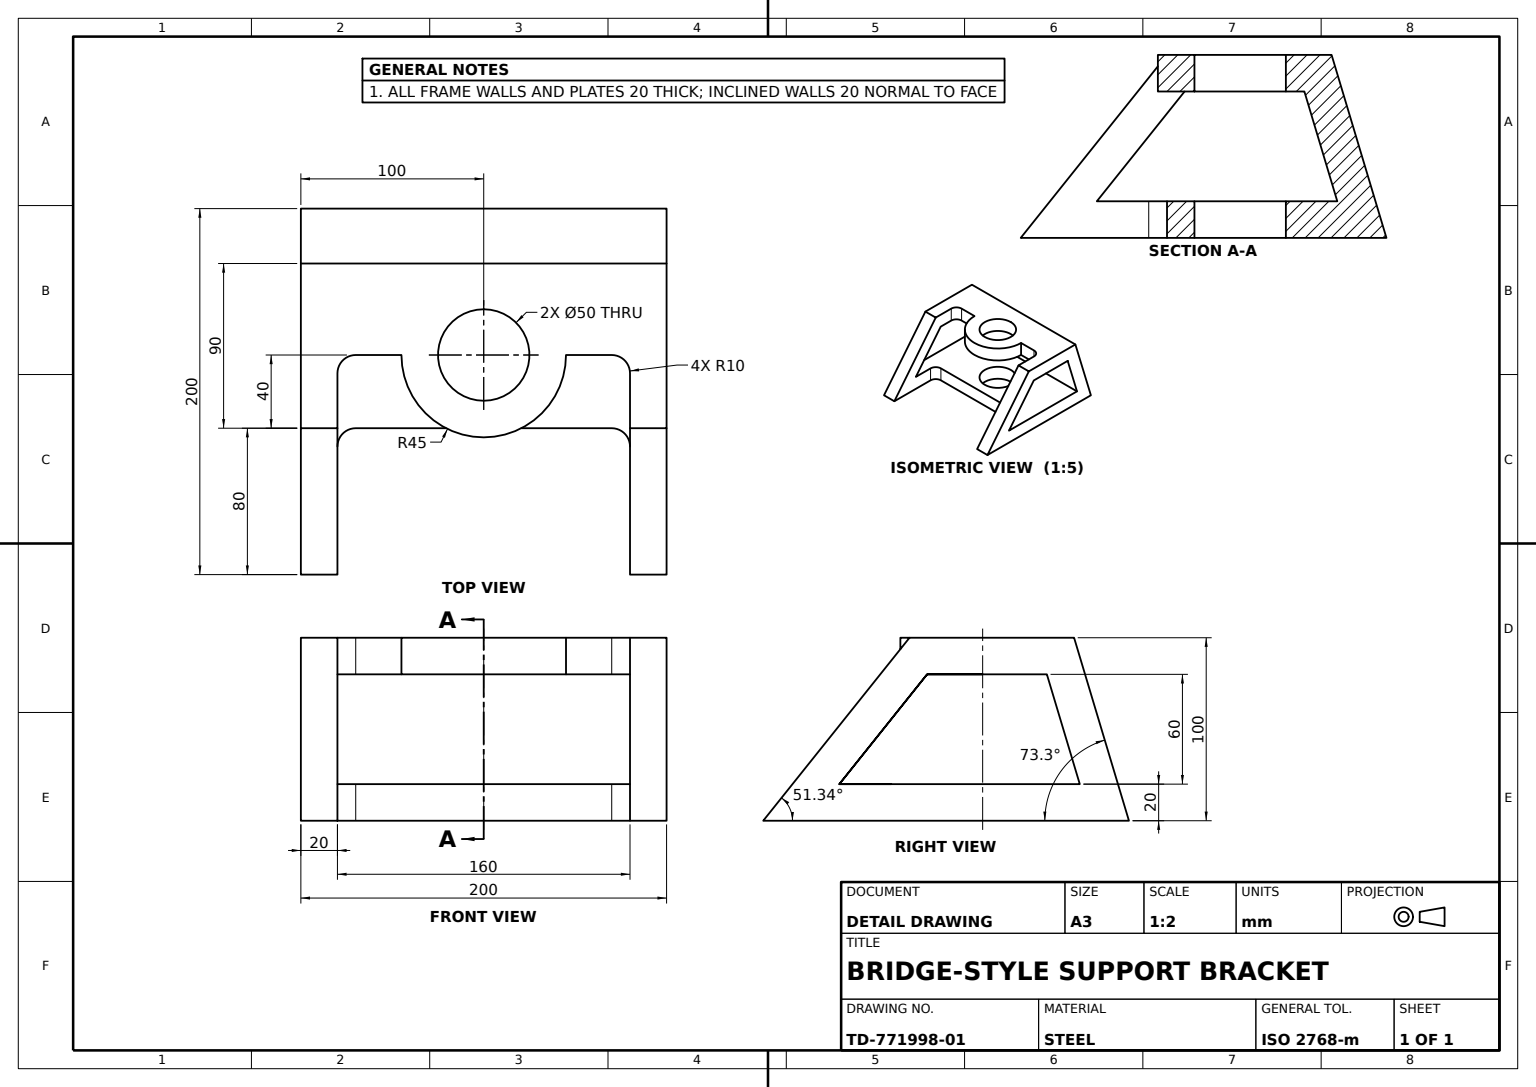
from build123d import *

# Parameters (mm, degrees)
FRAME_BODY_200_DEPTH        = 100
CENTRE_RECESS_SKETCH_W      = 160
CENTRE_RECESS_SKETCH_H      = 60
CENTRE_RECESS_CUT_DEPTH     = 150
WINDOW_A_CUT_REACH          = 246.949
WINDOW_A_SKETCH_80X60_W     = 160
WINDOW_A_SKETCH_80X60_H     = 60
WINDOW_B_CUT_REACH          = 239.487
WINDOW_B_SKETCH_W           = 160
WINDOW_B_SKETCH_H           = 80
WINDOW_CORNER_FILLETS_R10_R = 10
ANCHOR_BOSS_SKETCH_90_R     = 45
ANCHOR_BOSS_90_DEPTH        = 20
ANCHOR_BORE_SKETCH_50_R     = 25
ANCHOR_BORE_50_DEPTH        = 245.948974278


with BuildPart() as part:
    # Frame Profile Sketch → Frame Body 200 (new, symmetric)
    with BuildSketch(Plane(origin=(0, 0, 0), x_dir=(0, 0, -1), z_dir=(1, 0, 0))):
        Polygon((200, 0), (170, 100), (80, 100), (0, 0), align=None)
        Polygon((155.119386982, 80), (89.61249695, 80), (41.61249695, 20), (173.119386982, 20), align=None, mode=Mode.SUBTRACT)
    extrude(amount=FRAME_BODY_200_DEPTH, both=True)

    # Centre Recess Sketch → Centre Recess Cut (cut)
    with BuildSketch(Plane.XY):
        with Locations((0, 50)):
            Rectangle(CENTRE_RECESS_SKETCH_W, CENTRE_RECESS_SKETCH_H)
    extrude(amount=-CENTRE_RECESS_CUT_DEPTH, mode=Mode.SUBTRACT)

    # Window A Sketch 80x60 → Window A Cut (cut, up to next)
    with BuildSketch(Plane(origin=(0, 100, 0), x_dir=(1, 0, 0), z_dir=(0, 1, 0)), mode=Mode.PRIVATE) as window_a_cut_sk1:
        with Locations((0, 90)):
            Rectangle(WINDOW_A_SKETCH_80X60_W, WINDOW_A_SKETCH_80X60_H)
    window_a_cut_tool1 = extrude(window_a_cut_sk1.sketch, amount=-WINDOW_A_CUT_REACH, mode=Mode.PRIVATE) & part.part
    add(window_a_cut_tool1.solids().sort_by_distance((0, 100, -90))[0], mode=Mode.SUBTRACT)

    # Window B Sketch → Window B Cut (cut, up to next)
    with BuildSketch(Plane(origin=(0, 20, 0), x_dir=(1, 0, 0), z_dir=(0, 1, 0)), mode=Mode.PRIVATE) as window_b_cut_sk1:
        with Locations((0, 40)):
            Rectangle(WINDOW_B_SKETCH_W, WINDOW_B_SKETCH_H)
    window_b_cut_tool1 = extrude(window_b_cut_sk1.sketch, amount=-WINDOW_B_CUT_REACH, mode=Mode.PRIVATE) & part.part
    add(window_b_cut_tool1.solids().sort_by_distance((0, 20, -40))[0], mode=Mode.SUBTRACT)

    # Window Corner Fillets R10
    window_corner_fillets_r10_edges = [part.edges().sort_by_distance(p)[0] for p in [
        (80, 90, -120),
        (-80, 90, -120),
        (-80, 10, -80),
        (80, 10, -80),
    ]]
    fillet(window_corner_fillets_r10_edges, radius=WINDOW_CORNER_FILLETS_R10_R)

    # Anchor Boss Sketch Ø90 → Anchor Boss Ø90 (add)
    with BuildSketch(Plane(origin=(0, 100, 0), x_dir=(1, 0, 0), z_dir=(0, 1, 0))):
        with Locations((0, 120)):
            Circle(ANCHOR_BOSS_SKETCH_90_R)
    extrude(amount=-ANCHOR_BOSS_90_DEPTH)

    # Anchor Bore Sketch Ø50 → Anchor Bore Ø50 (cut, through all)
    with BuildSketch(Plane(origin=(0, 100, 0), x_dir=(1, 0, 0), z_dir=(0, 1, 0))):
        with Locations(Location((0, 120, 0), (0, 0, 270))):
            Circle(ANCHOR_BORE_SKETCH_50_R)
    extrude(amount=-ANCHOR_BORE_50_DEPTH, mode=Mode.SUBTRACT)


solid = part.part
